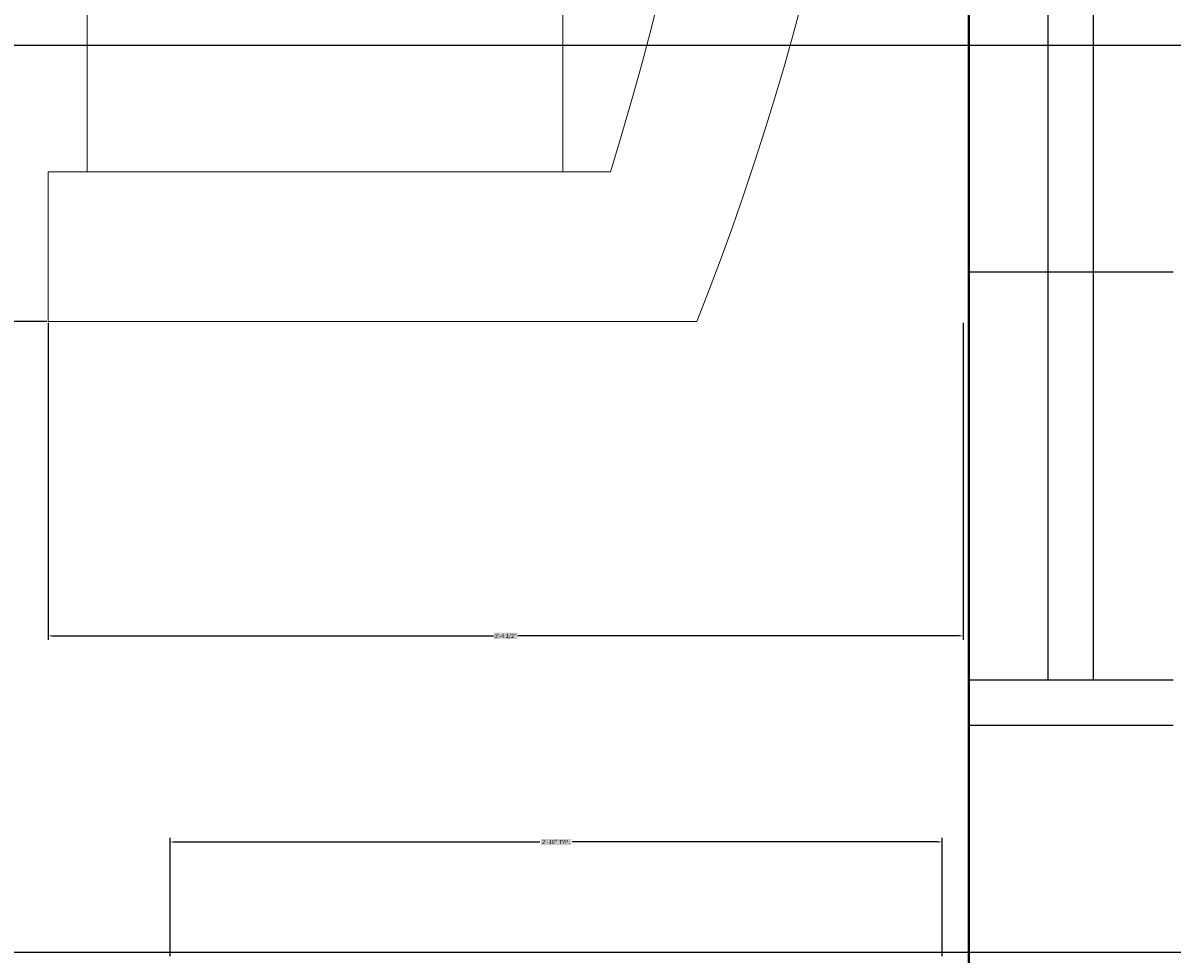
# Model space of a CAD drawing. Units: inches. Extents: x -301 to 715, y -607 to 364.
# Tile 102 of 141: x 82 to 133, y 26 to 67. Entities that reach past the tile are written whole.
import ezdxf

# ---------------------------------------------------------------- set-up
doc = ezdxf.new("R2010")
doc.units = ezdxf.units.IN
doc.header["$MEASUREMENT"] = 0
for name, color, linetype, lineweight in [('A-ANNO-DIMS', 2, 'Continuous', 18), ('A-FURN', 8, 'Continuous', 18), ('A-GLAZ', 2, 'Continuous', 25), ('A-WALL', 3, 'Continuous', 40)]:
    doc.layers.add(name, color=color, linetype=linetype, lineweight=lineweight)
doc.styles.get("Standard").update_dxf_attribs({"font": 'arial.ttf'})
doc.dimstyles.get("Standard").update_dxf_attribs({"dimtxt": 0.18, "dimasz": 0.18, "dimexe": 0.18, "dimexo": 0.0625, "dimgap": 0.09, "dimtad": 0, "dimtih": 1, "dimtoh": 1, "dimdec": 1, "dimzin": 0, "dimdsep": 46, "dimlunit": 4, "dimtxsty": 'Standard', "dimcen": 0.09, "dimclrd": 3, "dimclre": 4, "dimclrt": 6, "dimadec": 0, "dimazin": 0, "dimtfac": 1, "dimtdec": 1, "dimtofl": 0, "dimtmove": 0, "dimatfit": 3, "dimfxl": 1, "dimtfill": 2, "dimtfillclr": 51, "dimtolj": 1, "dimtzin": 0, "dimarcsym": 0})

# ---------------------------------------------------------------- blocks, each defined once
blk = doc.blocks.new('Sofa - Roundback 7 ft.')
for p, q in [((35.99998, -34), (35.99998, -11.4696)), ((-35.999844, -13.3819), (35.9998, -13.3819)), ((-36.000027, -32.4421), (35.99998, -32.4421))]:
    blk.add_line(p, q)
blk.add_lwpolyline([(41.99998, -8), (41.99998, -34), (35.99998, -34)])
for centre, radius, start, end in [((0, -114.25), 114.25, 68.43141, 111.5686), ((-0.00001, -127.1968), 121.1968, 72.72033, 107.2797)]:
    blk.add_arc(centre, radius, start, end)
blk = doc.blocks.new('WIN-36-PLAN')
for p, q in [((0, 0), (0, 9)), ((2, 0), (2, 9)), ((20, 0), (20, 9)), ((38, 0), (38, 9)), ((40, 0), (40, 9)), ((2, 5.5), (38, 5.5)), ((2, 3.5), (38, 3.5))]:
    blk.add_line(p, q)
blk = doc.blocks.new('*D119')
at = {"layer": 'A-ANNO-DIMS', "color": 4, "lineweight": -2, "transparency": 16777216}
for p, q in [((88.66, 25.504), (88.66, 30.729)), ((122.71, 25.504), (122.71, 30.729))]:
    blk.add_line(p, q, dxfattribs=at)
at = {"layer": 'A-ANNO-DIMS', "color": 3, "lineweight": -2, "transparency": 16777216}
for p, q in [((88.84, 30.549), (104.975, 30.549)), ((122.53, 30.549), (106.395, 30.549))]:
    blk.add_line(p, q, dxfattribs=at)
at = {"layer": 'A-ANNO-DIMS', "color": 3, "transparency": 16777216}
for points in [[(88.84, 30.579), (88.84, 30.519), (88.66, 30.549)], [(122.53, 30.579), (122.53, 30.519), (122.71, 30.549)]]:
    blk.add_solid(points, dxfattribs=at)
at = {"layer": 'Defpoints', "color": 0, "transparency": 16777216}
for p in [(122.71, 30.549), (88.66, 25.442), (122.71, 25.442)]:
    blk.add_point(p, dxfattribs=at)
at = {"layer": 'A-ANNO-DIMS', "color": 6, "transparency": 16777216, "insert": (105.685, 30.549), "char_height": 0.18, "attachment_point": 5, "bg_fill": 1, "box_fill_scale": 1.25, "bg_fill_color": 51, "bg_fill_transparency": 0}
blk.add_mtext('\\A1;2\'-10" TYP.', dxfattribs=at)
blk = doc.blocks.new('*D132')
at = {"layer": 'A-ANNO-DIMS', "color": 4, "lineweight": -2, "transparency": 16777216}
for p, q in [((83.224, 145.954), (69.239, 145.954)), ((83.224, 53.504), (69.239, 53.504))]:
    blk.add_line(p, q, dxfattribs=at)
at = {"layer": 'A-ANNO-DIMS', "color": 3, "lineweight": -2, "transparency": 16777216}
for p, q in [((69.419, 145.774), (69.419, 99.912)), ((69.419, 53.684), (69.419, 99.546))]:
    blk.add_line(p, q, dxfattribs=at)
at = {"layer": 'A-ANNO-DIMS', "color": 3, "transparency": 16777216}
for points in [[(69.389, 145.774), (69.449, 145.774), (69.419, 145.954)], [(69.389, 53.684), (69.449, 53.684), (69.419, 53.504)]]:
    blk.add_solid(points, dxfattribs=at)
at = {"layer": 'Defpoints', "color": 0, "transparency": 16777216}
for p in [(83.287, 145.954), (69.419, 53.504), (83.287, 53.504)]:
    blk.add_point(p, dxfattribs=at)
at = {"layer": 'A-ANNO-DIMS', "color": 6, "transparency": 16777216, "insert": (69.419, 99.729), "char_height": 0.18, "attachment_point": 5, "bg_fill": 1, "box_fill_scale": 1.25, "bg_fill_color": 51, "bg_fill_transparency": 0}
blk.add_mtext('\\A1;SOFA 7\'-8 1/2"', dxfattribs=at)
blk = doc.blocks.new('*D133')
at = {"layer": 'A-ANNO-DIMS', "color": 4, "lineweight": -2, "transparency": 16777216}
for p, q in [((83.287, 53.442), (83.287, 39.457)), ((123.642, 53.442), (123.642, 39.457))]:
    blk.add_line(p, q, dxfattribs=at)
at = {"layer": 'A-ANNO-DIMS', "color": 3, "lineweight": -2, "transparency": 16777216}
for p, q in [((83.467, 39.637), (102.925, 39.637)), ((123.462, 39.637), (104.003, 39.637))]:
    blk.add_line(p, q, dxfattribs=at)
at = {"layer": 'A-ANNO-DIMS', "color": 3, "transparency": 16777216}
for points in [[(83.467, 39.667), (83.467, 39.607), (83.287, 39.637)], [(123.462, 39.667), (123.462, 39.607), (123.642, 39.637)]]:
    blk.add_solid(points, dxfattribs=at)
at = {"layer": 'Defpoints', "color": 0, "transparency": 16777216}
for p in [(83.287, 53.504), (123.642, 53.504), (123.642, 39.637)]:
    blk.add_point(p, dxfattribs=at)
at = {"layer": 'A-ANNO-DIMS', "color": 6, "transparency": 16777216, "insert": (103.464, 39.637), "char_height": 0.18, "attachment_point": 5, "bg_fill": 1, "box_fill_scale": 1.25, "bg_fill_color": 51, "bg_fill_transparency": 0}
blk.add_mtext('\\A1;3\'-4 1/2"', dxfattribs=at)
blk = doc.blocks.new('*D149')
at = {"layer": 'A-ANNO-DIMS', "color": 4, "lineweight": -2, "transparency": 16777216}
for p, q in [((-51.541, 65.682), (233.659, 65.682)), ((-51.541, 25.682), (233.659, 25.682))]:
    blk.add_line(p, q, dxfattribs=at)
at = {"layer": 'A-ANNO-DIMS', "color": 3, "lineweight": -2, "transparency": 16777216}
for p, q in [((233.479, 65.502), (233.479, 45.864)), ((233.479, 25.862), (233.479, 45.5))]:
    blk.add_line(p, q, dxfattribs=at)
at = {"layer": 'A-ANNO-DIMS', "color": 3, "transparency": 16777216}
for points in [[(233.449, 65.502), (233.509, 65.502), (233.479, 65.682)], [(233.449, 25.862), (233.509, 25.862), (233.479, 25.682)]]:
    blk.add_solid(points, dxfattribs=at)
at = {"layer": 'Defpoints', "color": 0, "transparency": 16777216}
for p in [(-51.603, 65.682), (-51.603, 25.682), (233.479, 25.682)]:
    blk.add_point(p, dxfattribs=at)
at = {"layer": 'A-ANNO-DIMS', "color": 6, "transparency": 16777216, "insert": (233.479, 45.682), "char_height": 0.18, "attachment_point": 5, "bg_fill": 1, "box_fill_scale": 1.25, "bg_fill_color": 51, "bg_fill_transparency": 0}
blk.add_mtext('\\A1;3\'-4"', dxfattribs=at)

msp = doc.modelspace()

# ---------------------------------------------------------------- linework, layer by layer
at = {"layer": 'A-WALL'}
msp.add_line((123.897, -9.818), (123.897, 193.182), dxfattribs=at)

# ---------------------------------------------------------------- block references
at = {"layer": 'A-FURN', "xscale": 1.100593323052692, "yscale": 1.100593323052692, "zscale": 1.100593323052692, "rotation": 270}
msp.add_blockref('Sofa - Roundback 7 ft.', (120.707, 99.729), dxfattribs=at)
at = {"layer": 'A-GLAZ', "rotation": 90.00000000000036}
msp.add_blockref('WIN-36-PLAN', (132.897, 35.683), dxfattribs=at)

# ---------------------------------------------------------------- dimensions: what is measured, and where the dimension line sits
at = {"layer": 'A-ANNO-DIMS'}
dim = msp.add_linear_dim(base=(69.4192, 53.5044), p1=(83.2867, 145.9543), p2=(83.2867, 53.5044), angle=270, text='SOFA <>', dimstyle='Standard', override={"dimdec": 1, "dimlfac": 1, "dimrnd": 0, "dimzin": 1, "dimdsep": 46, "dimlunit": 4, "dimfrac": 2}, dxfattribs=at)
dim.commit()
dim.dimension.update_dxf_attribs({"geometry": '*D132', "text_midpoint": (69.4192, 99.7293)})
dim = msp.add_linear_dim(base=(233.479, 25.682), p1=(-51.603, 65.682), p2=(-51.603, 25.682), angle=90, dimstyle='Standard', override={"dimdec": 1, "dimlfac": 1, "dimrnd": 0, "dimzin": 1, "dimdsep": 46, "dimlunit": 4, "dimfrac": 2}, dxfattribs=at)
dim.commit()
dim.dimension.update_dxf_attribs({"geometry": '*D149', "text_midpoint": (233.479, 45.682)})
dim = msp.add_linear_dim(base=(123.642, 39.637), p1=(83.287, 53.504), p2=(123.642, 53.504), dimstyle='Standard', override={"dimdec": 1, "dimlfac": 1, "dimrnd": 0, "dimzin": 1, "dimdsep": 46, "dimlunit": 4, "dimfrac": 2}, dxfattribs=at)
dim.commit()
dim.dimension.update_dxf_attribs({"geometry": '*D133', "text_midpoint": (103.464, 39.637)})
dim = msp.add_linear_dim(base=(122.7099, 30.5493), p1=(88.6597, 25.4415), p2=(122.7099, 25.4415), text='<> TYP.', dimstyle='Standard', override={"dimdec": 1, "dimlfac": 1, "dimrnd": 0, "dimzin": 1, "dimdsep": 46, "dimlunit": 4, "dimfrac": 2}, dxfattribs=at)
dim.commit()
dim.dimension.update_dxf_attribs({"geometry": '*D119', "text_midpoint": (105.6848, 30.5493)})

doc.saveas('drawing.dxf')
